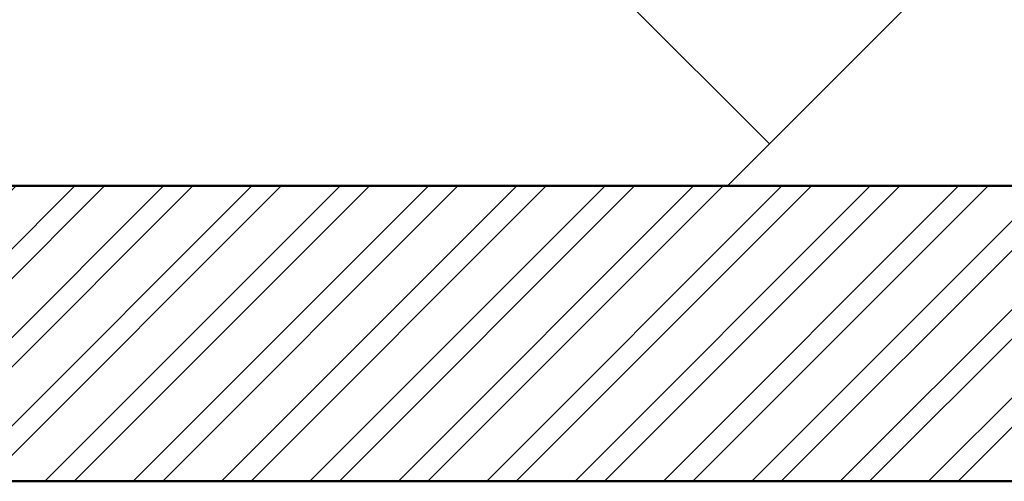
# Model space of a CAD drawing. Units: inches. Extents: x 3590 to 5167, y 65 to 1917.
# Tile 38 of 100: x 5035 to 5065, y 1326 to 1340. Entities that reach past the tile are written whole.
import ezdxf

# ---------------------------------------------------------------- set-up
doc = ezdxf.new("R2010")
doc.units = ezdxf.units.IN
for name, color, linetype, lineweight in [('A-FLOR-PATT', 8, 'Continuous', 13), ('A-WALL', 7, 'Continuous', 50), ('A-WALL-PATT', 251, 'Continuous', 13)]:
    doc.layers.add(name, color=color, linetype=linetype, lineweight=lineweight)

msp = doc.modelspace()

# ---------------------------------------------------------------- hatches: boundary and pattern name
at = {"layer": 'A-FLOR-PATT', "transparency": 33554687}
h = msp.add_hatch(dxfattribs=at)
h.set_pattern_fill('AR-HBONE', color=256, scale=0.2)
h.set_pattern_definition([(45, (-588.972, 0), (0, 28.73682), [60.96, -20.32]), (135, (-574.604, 14.368), (3e-15, 28.73682), [60.96, -20.32])])
h.paths.add_polyline_path([(5071.274, 1796.999), (4933.274, 1796.999), (4933.274, 1753.999), (4962.774, 1753.999, -0.414214), (4928.774, 1719.999), (4933.274, 1718.999), (4933.274, 1334.999), (5071.274, 1334.999)])
h.paths.add_polyline_path([(4951.78, 1521.077), (4951.715, 1521.04), (4951.563, 1520.895)], flags=16)
h.paths.add_polyline_path([(4952.267, 1521.376), (4952.198, 1521.371), (4952.198, 1521.356)], flags=0)
h.paths.add_polyline_path([(4967.051, 1529.728), (4965.231, 1528.694), (4963.411, 1527.714), (4961.756, 1526.851), (4963.589, 1527.449), (4964.036, 1527.478), (4962.975, 1527.249), (4961.76, 1526.852), (4959.792, 1525.834), (4958.005, 1524.895), (4956.24, 1523.93), (4954.504, 1522.919), (4954.129, 1522.682), (4953.361, 1521.997), (4953.366, 1521.998), (4953.605, 1522.064), (4955.106, 1522.761), (4956.921, 1523.434), (4958.678, 1523.915), (4960.358, 1524.2), (4961.945, 1524.286), (4964.171, 1524.108), (4965.958, 1523.309), (4963.863, 1522.976), (4965.187, 1522.499), (4963.366, 1522.497), (4961.545, 1522.487), (4959.764, 1522.461), (4958.304, 1522.419), (4957.974, 1522.388), (4956.307, 1522.232), (4954.718, 1522.071), (4953.251, 1521.899), (4953.525, 1521.623), (4954.331, 1521.379), (4956.243, 1521.23), (4958.039, 1520.93), (4959.684, 1520.483), (4961.16, 1519.896), (4963.107, 1518.8), (4964.393, 1517.325), (4962.973, 1517.726), (4964.558, 1516.661), (4965.407, 1515.708), (4963.507, 1516.322), (4961.68, 1517.005), (4959.935, 1517.745), (4958.282, 1518.528), (4956.732, 1519.343), (4955.295, 1520.175), (4954.672, 1520.572), (4954.513, 1520.627), (4955.658, 1519.318), (4956.703, 1517.982), (4957.644, 1516.647), (4958.485, 1515.334), (4959.55, 1513.524), (4960.438, 1511.769), (4958.841, 1513.62), (4957.452, 1515.325), (4955.819, 1517.459), (4956.665, 1515.448), (4957.111, 1513.923), (4957.447, 1511.714), (4957.076, 1509.793), (4956.538, 1511.11), (4955.992, 1512.569), (4955.444, 1514.125), (4954.898, 1515.735), (4954.357, 1517.356), (4953.824, 1518.943), (4953.305, 1520.452), (4953.065, 1521.116), (4952.971, 1521.146), (4952.949, 1521.086), (4952.73, 1520.199), (4953.37, 1518.024), (4953.757, 1516.373), (4954.051, 1514.765), (4954.264, 1513.221), (4954.471, 1511.131), (4954.497, 1510.402), (4954.409, 1511.76), (4954.264, 1513.221), (4954.051, 1514.765), (4953.757, 1516.373), (4953.37, 1518.024), (4952.877, 1519.698), (4952.716, 1520.141), (4952.533, 1519.059), (4952.374, 1517.789), (4952.219, 1516.312), (4952.046, 1514.6), (4951.833, 1512.626), (4951.557, 1510.363), (4951.203, 1512.168), (4950.852, 1514.339), (4950.985, 1516.376), (4951.66, 1518.286), (4952.593, 1520.481), (4952.357, 1521.13), (4951.855, 1520.328), (4950.839, 1518.908), (4949.777, 1517.587), (4948.916, 1516.617), (4948.111, 1515.256), (4947.089, 1513.554), (4945.889, 1511.615), (4946.326, 1513.402), (4946.562, 1514.249), (4945.528, 1513.327), (4944.581, 1512.531), (4946.018, 1514.508), (4947.204, 1516.048), (4947.893, 1517.313), (4949.307, 1518.764), (4950.414, 1519.767), (4950.451, 1519.806), (4952.267, 1521.376), (4951.645, 1521.493), (4950.404, 1521.18), (4948.044, 1520.359), (4946.119, 1519.452), (4944.572, 1518.475), (4943.35, 1517.443), (4941.997, 1515.92), (4941.661, 1515.275), (4942.813, 1516.99), (4944.572, 1518.475), (4946.119, 1519.452), (4948.044, 1520.359), (4950.404, 1521.18), (4951.645, 1521.493), (4949.647, 1521.868), (4948.6, 1521.756), (4947.126, 1521.57), (4945.42, 1521.348), (4943.45, 1521.105), (4941.183, 1520.856), (4942.86, 1521.613), (4943.873, 1522.03), (4942.952, 1521.909), (4941.41, 1521.485), (4939.543, 1520.67), (4938.968, 1520.226), (4940.733, 1521.299), (4942.952, 1521.909), (4943.702, 1522.008), (4945.894, 1522.7), (4947.565, 1522.714), (4948.921, 1522.566), (4951.131, 1522.183), (4950.971, 1522.297), (4948.129, 1523.006), (4946.035, 1523.707), (4944.232, 1524.521), (4942.707, 1525.461), (4941.444, 1526.537), (4940.43, 1527.761), (4939.649, 1529.143), (4941.421, 1528.122), (4943.147, 1527.132), (4944.841, 1526.175), (4946.514, 1525.25), (4948.179, 1524.359), (4948.365, 1524.263), (4946.475, 1526.045), (4945.181, 1527.54), (4944.19, 1529.033), (4943.496, 1530.54), (4943.278, 1531.36), (4942.498, 1531.919), (4943.114, 1531.762), (4942.959, 1533.659), (4944.14, 1531.989), (4944.612, 1531.323), (4946.202, 1530.463), (4947.486, 1529.509), (4948.79, 1528.226), (4950.368, 1526.237), (4949.485, 1528.155), (4948.851, 1530.123), (4948.491, 1532.041), (4948.381, 1533.918), (4948.501, 1535.76), (4948.827, 1537.573), (4949.418, 1535.565), (4949.957, 1533.569), (4950.464, 1531.586), (4950.961, 1529.617), (4951.391, 1527.954), (4951.724, 1530.687), (4952.201, 1532.58), (4952.889, 1534.33), (4953.77, 1535.951), (4954.827, 1537.46), (4954.521, 1535.39), (4954.273, 1533.937), (4955.58, 1535.663), (4956.748, 1536.739), (4956.159, 1534.78), (4955.589, 1532.873), (4955.043, 1531.006), (4954.525, 1529.166), (4954.038, 1527.341), (4953.638, 1525.733), (4953.611, 1525.586), (4953.398, 1524.166), (4953.382, 1524.009), (4954.07, 1525.476), (4954.912, 1527.022), (4956.136, 1528.894), (4957.847, 1530.577), (4959.376, 1531.54), (4958.256, 1530.104), (4957.143, 1528.663), (4956.066, 1527.243), (4955.056, 1525.871), (4954.141, 1524.571), (4953.352, 1523.372), (4953.311, 1523.303), (4953.273, 1522.925), (4953.261, 1522.382), (4954.103, 1523.373), (4954.63, 1524.284), (4955.961, 1526.358), (4957.23, 1528.13), (4958.421, 1529.609), (4960.037, 1531.368), (4961.374, 1532.375), (4962.101, 1532.77), (4961.07, 1531.061), (4959.987, 1529.438), (4958.869, 1527.908), (4958.15, 1527.007), (4959.803, 1528.003), (4961.589, 1528.793), (4963.391, 1529.328), (4965.211, 1529.632)], flags=16)
h.paths.add_polyline_path([(4962.944, 1523.182), (4961.107, 1523.422), (4960.392, 1523.362), (4962.35, 1523.331)], flags=0)
h.paths.add_polyline_path([(5049.541, 1584.551), (5049.476, 1584.515), (5049.325, 1584.37)], flags=16)
h.paths.add_polyline_path([(5050.028, 1584.851), (5049.959, 1584.845), (5049.959, 1584.83)], flags=0)
h.paths.add_polyline_path([(5042.333, 1581.949), (5043.88, 1582.926), (5045.806, 1583.833), (5048.165, 1584.654), (5049.406, 1584.967), (5047.408, 1585.342), (5046.361, 1585.231), (5044.888, 1585.044), (5043.181, 1584.822), (5041.211, 1584.579), (5038.944, 1584.33), (5040.622, 1585.087), (5041.634, 1585.504), (5040.713, 1585.383), (5039.171, 1584.959), (5037.304, 1584.144), (5036.729, 1583.7), (5038.494, 1584.773), (5040.713, 1585.383), (5041.463, 1585.482), (5043.655, 1586.174), (5045.326, 1586.188), (5046.682, 1586.04), (5048.893, 1585.657), (5048.732, 1585.771), (5045.891, 1586.48), (5043.796, 1587.181), (5041.994, 1587.996), (5040.468, 1588.935), (5039.205, 1590.011), (5038.191, 1591.235), (5037.41, 1592.617), (5039.182, 1591.596), (5040.909, 1590.607), (5042.602, 1589.649), (5044.275, 1588.724), (5045.94, 1587.833), (5046.126, 1587.738), (5044.237, 1589.519), (5042.942, 1591.015), (5041.952, 1592.508), (5041.257, 1594.014), (5041.039, 1594.834), (5040.26, 1595.393), (5040.875, 1595.237), (5040.721, 1597.133), (5041.901, 1595.463), (5042.373, 1594.798), (5043.963, 1593.938), (5045.247, 1592.983), (5046.552, 1591.701), (5048.129, 1589.712), (5047.247, 1591.63), (5046.613, 1593.597), (5046.252, 1595.515), (5046.142, 1597.392), (5046.262, 1599.234), (5046.588, 1601.047), (5047.179, 1599.039), (5047.718, 1597.043), (5048.225, 1595.06), (5048.722, 1593.091), (5049.152, 1591.429), (5049.485, 1594.161), (5049.962, 1596.054), (5050.65, 1597.804), (5051.532, 1599.425), (5052.589, 1600.934), (5052.283, 1598.864), (5052.034, 1597.411), (5053.341, 1599.137), (5054.509, 1600.213), (5053.92, 1598.254), (5053.35, 1596.348), (5052.805, 1594.48), (5052.286, 1592.64), (5051.799, 1590.815), (5051.4, 1589.207), (5051.373, 1589.06), (5051.159, 1587.64), (5051.143, 1587.483), (5051.831, 1588.95), (5052.673, 1590.496), (5053.898, 1592.368), (5055.608, 1594.051), (5057.137, 1595.014), (5056.017, 1593.578), (5054.904, 1592.137), (5053.828, 1590.717), (5052.817, 1589.345), (5051.902, 1588.046), (5051.113, 1586.846), (5051.072, 1586.777), (5051.034, 1586.399), (5051.022, 1585.856), (5051.864, 1586.847), (5052.391, 1587.758), (5053.723, 1589.832), (5054.991, 1591.604), (5056.182, 1593.083), (5057.798, 1594.842), (5059.135, 1595.849), (5059.863, 1596.244), (5058.831, 1594.535), (5057.749, 1592.912), (5056.63, 1591.382), (5055.912, 1590.482), (5057.564, 1591.477), (5059.35, 1592.267), (5061.152, 1592.802), (5062.972, 1593.106), (5064.812, 1593.203), (5062.992, 1592.169), (5061.172, 1591.188), (5059.518, 1590.325), (5061.35, 1590.924), (5061.797, 1590.952), (5060.737, 1590.723), (5059.521, 1590.326), (5057.553, 1589.308), (5055.766, 1588.369), (5054.002, 1587.404), (5052.265, 1586.393), (5051.891, 1586.156), (5051.122, 1585.471), (5051.127, 1585.472), (5051.366, 1585.538), (5052.867, 1586.235), (5054.682, 1586.908), (5056.439, 1587.389), (5058.12, 1587.675), (5059.706, 1587.76), (5061.933, 1587.583), (5063.719, 1586.783), (5061.624, 1586.45), (5062.949, 1585.973), (5061.127, 1585.971), (5059.307, 1585.961), (5057.525, 1585.935), (5056.065, 1585.893), (5055.735, 1585.862), (5054.068, 1585.707), (5052.479, 1585.546), (5051.012, 1585.373), (5051.286, 1585.097), (5052.092, 1584.853), (5054.004, 1584.704), (5055.8, 1584.404), (5057.446, 1583.958), (5058.921, 1583.37), (5060.868, 1582.274), (5062.154, 1580.799), (5060.734, 1581.2), (5062.32, 1580.135), (5063.168, 1579.182), (5061.269, 1579.796), (5059.441, 1580.479), (5057.696, 1581.219), (5056.043, 1582.003), (5054.493, 1582.817), (5053.057, 1583.649), (5052.433, 1584.047), (5052.274, 1584.101), (5053.42, 1582.793), (5054.464, 1581.457), (5055.405, 1580.121), (5056.247, 1578.809), (5057.311, 1576.998), (5058.199, 1575.244), (5056.602, 1577.094), (5055.213, 1578.799), (5053.58, 1580.933), (5054.427, 1578.922), (5054.872, 1577.397), (5055.208, 1575.189), (5054.838, 1573.267), (5054.299, 1574.584), (5053.754, 1576.043), (5053.206, 1577.599), (5052.659, 1579.209), (5052.118, 1580.83), (5051.585, 1582.417), (5051.066, 1583.927), (5050.826, 1584.59), (5050.733, 1584.62), (5050.711, 1584.561), (5050.491, 1583.673), (5051.131, 1581.498), (5051.518, 1579.847), (5051.813, 1578.24), (5052.026, 1576.695), (5052.233, 1574.605), (5052.258, 1573.876), (5052.17, 1575.234), (5052.026, 1576.695), (5051.813, 1578.24), (5051.518, 1579.847), (5051.131, 1581.498), (5050.638, 1583.172), (5050.477, 1583.615), (5050.294, 1582.533), (5050.136, 1581.263), (5049.981, 1579.786), (5049.807, 1578.074), (5049.594, 1576.1), (5049.318, 1573.837), (5048.965, 1575.642), (5048.613, 1577.813), (5048.747, 1579.85), (5049.421, 1581.76), (5050.354, 1583.955), (5050.118, 1584.604), (5049.616, 1583.802), (5048.6, 1582.382), (5047.538, 1581.061), (5046.677, 1580.091), (5045.872, 1578.73), (5044.85, 1577.028), (5043.651, 1575.089), (5044.087, 1576.877), (5044.324, 1577.723), (5043.289, 1576.801), (5042.342, 1576.005), (5043.779, 1577.982), (5044.966, 1579.522), (5045.655, 1580.787), (5047.068, 1582.239), (5048.175, 1583.241), (5048.213, 1583.28), (5050.028, 1584.851), (5049.406, 1584.967), (5048.165, 1584.654), (5045.806, 1583.833), (5043.88, 1582.926), (5042.333, 1581.949), (5041.111, 1580.917), (5039.758, 1579.394), (5039.423, 1578.749), (5040.575, 1580.464)], flags=16)
h.paths.add_polyline_path([(4954.799, 1533.12), (4954.262, 1532.079), (4953.831, 1530.935), (4953.505, 1529.636), (4953.283, 1528.133), (4953.167, 1526.376), (4953.156, 1524.315), (4953.277, 1521.236), (4952.802, 1521.842), (4951.557, 1521.998), (4950.976, 1521.961), (4952.661, 1521.941), (4952.802, 1521.842), (4953.152, 1523.593), (4953.167, 1526.376), (4953.283, 1528.133), (4953.609, 1530.346), (4954.456, 1532.592)], flags=0)
h.paths.add_polyline_path([(5050.563, 1585.316), (5049.318, 1585.472), (5048.737, 1585.435), (5050.422, 1585.415), (5050.563, 1585.316), (5050.914, 1587.067), (5050.928, 1589.851), (5051.045, 1591.607), (5051.371, 1593.82), (5052.217, 1596.066), (5052.56, 1596.594), (5052.024, 1595.554), (5051.592, 1594.409), (5051.266, 1593.11), (5051.045, 1591.607), (5050.928, 1589.851), (5050.918, 1587.789), (5051.038, 1584.71)], flags=0)
h.paths.add_polyline_path([(5058.153, 1586.836), (5060.111, 1586.805), (5060.705, 1586.656), (5058.868, 1586.896)], flags=0)
h.paths.add_polyline_path([(5049.541, 1430.936), (5049.476, 1430.9), (5049.325, 1430.755)], flags=16)
h.paths.add_polyline_path([(5050.028, 1431.236), (5049.959, 1431.231), (5049.959, 1431.215)], flags=0)
h.paths.add_polyline_path([(5046.588, 1447.432), (5047.179, 1445.425), (5047.718, 1443.429), (5048.225, 1441.446), (5048.722, 1439.476), (5049.152, 1437.814), (5049.485, 1440.546), (5049.962, 1442.439), (5050.65, 1444.189), (5051.532, 1445.811), (5052.589, 1447.319), (5052.283, 1445.249), (5052.034, 1443.796), (5053.341, 1445.522), (5054.509, 1446.598), (5053.92, 1444.64), (5053.35, 1442.733), (5052.805, 1440.865), (5052.286, 1439.025), (5051.799, 1437.201), (5051.4, 1435.592), (5051.373, 1435.445), (5051.159, 1434.025), (5051.143, 1433.868), (5051.831, 1435.335), (5052.673, 1436.881), (5053.898, 1438.753), (5055.608, 1440.436), (5057.137, 1441.4), (5056.017, 1439.963), (5054.904, 1438.522), (5053.828, 1437.102), (5052.817, 1435.73), (5051.902, 1434.431), (5051.113, 1433.231), (5051.072, 1433.162), (5051.034, 1432.784), (5051.022, 1432.242), (5051.864, 1433.232), (5052.391, 1434.143), (5053.723, 1436.217), (5054.991, 1437.989), (5056.182, 1439.468), (5057.798, 1441.227), (5059.135, 1442.235), (5059.863, 1442.629), (5058.831, 1440.921), (5057.749, 1439.298), (5056.63, 1437.767), (5055.912, 1436.867), (5057.564, 1437.863), (5059.35, 1438.652), (5061.152, 1439.187), (5062.972, 1439.491), (5064.812, 1439.588), (5062.992, 1438.554), (5061.172, 1437.573), (5059.518, 1436.71), (5061.35, 1437.309), (5061.797, 1437.337), (5060.737, 1437.108), (5059.521, 1436.711), (5057.553, 1435.693), (5055.766, 1434.754), (5054.002, 1433.789), (5052.265, 1432.778), (5051.891, 1432.541), (5051.122, 1431.856), (5051.127, 1431.857), (5051.366, 1431.923), (5052.867, 1432.62), (5054.682, 1433.293), (5056.439, 1433.775), (5058.12, 1434.06), (5059.706, 1434.145), (5061.933, 1433.968), (5063.719, 1433.168), (5061.624, 1432.835), (5062.949, 1432.358), (5061.127, 1432.357), (5059.307, 1432.346), (5057.525, 1432.32), (5056.065, 1432.278), (5055.735, 1432.248), (5054.068, 1432.092), (5052.479, 1431.931), (5051.012, 1431.759), (5051.286, 1431.482), (5052.092, 1431.238), (5054.004, 1431.089), (5055.8, 1430.789), (5057.446, 1430.343), (5058.921, 1429.755), (5060.868, 1428.66), (5062.154, 1427.185), (5060.734, 1427.585), (5062.32, 1426.52), (5063.168, 1425.567), (5061.269, 1426.181), (5059.441, 1426.865), (5057.696, 1427.604), (5056.043, 1428.388), (5054.493, 1429.202), (5053.057, 1430.034), (5052.433, 1430.432), (5052.274, 1430.487), (5053.42, 1429.178), (5054.464, 1427.842), (5055.405, 1426.506), (5056.247, 1425.194), (5057.311, 1423.383), (5058.199, 1421.629), (5056.602, 1423.479), (5055.213, 1425.184), (5053.58, 1427.318), (5054.427, 1425.307), (5054.872, 1423.782), (5055.208, 1421.574), (5054.838, 1419.652), (5054.299, 1420.97), (5053.754, 1422.428), (5053.206, 1423.984), (5052.659, 1425.595), (5052.118, 1427.215), (5051.585, 1428.802), (5051.066, 1430.312), (5050.826, 1430.975), (5050.733, 1431.005), (5050.711, 1430.946), (5050.491, 1430.058), (5051.131, 1427.883), (5051.518, 1426.232), (5051.813, 1424.625), (5052.026, 1423.081), (5052.233, 1420.991), (5052.258, 1420.261), (5052.17, 1421.619), (5052.026, 1423.081), (5051.813, 1424.625), (5051.518, 1426.232), (5051.131, 1427.883), (5050.638, 1429.558), (5050.477, 1430.001), (5050.294, 1428.918), (5050.136, 1427.648), (5049.981, 1426.171), (5049.807, 1424.459), (5049.594, 1422.485), (5049.318, 1420.222), (5048.965, 1422.028), (5048.613, 1424.199), (5048.747, 1426.235), (5049.421, 1428.146), (5050.354, 1430.34), (5050.118, 1430.989), (5049.616, 1430.187), (5048.6, 1428.768), (5047.538, 1427.446), (5046.677, 1426.477), (5045.872, 1425.116), (5044.85, 1423.413), (5043.651, 1421.474), (5044.087, 1423.262), (5044.324, 1424.109), (5043.289, 1423.186), (5042.342, 1422.391), (5043.779, 1424.368), (5044.966, 1425.907), (5045.655, 1427.173), (5047.068, 1428.624), (5048.175, 1429.627), (5048.213, 1429.666), (5050.028, 1431.236), (5049.406, 1431.353), (5048.165, 1431.039), (5045.806, 1430.218), (5043.88, 1429.311), (5042.333, 1428.334), (5041.111, 1427.302), (5039.758, 1425.779), (5039.423, 1425.134), (5040.575, 1426.849), (5042.333, 1428.334), (5043.88, 1429.311), (5045.806, 1430.218), (5048.165, 1431.039), (5049.406, 1431.353), (5047.408, 1431.727), (5046.361, 1431.616), (5044.888, 1431.429), (5043.181, 1431.207), (5041.211, 1430.964), (5038.944, 1430.715), (5040.622, 1431.472), (5041.634, 1431.89), (5040.713, 1431.769), (5039.171, 1431.345), (5037.304, 1430.53), (5036.729, 1430.085), (5038.494, 1431.158), (5040.713, 1431.769), (5041.463, 1431.867), (5043.655, 1432.559), (5045.326, 1432.573), (5046.682, 1432.425), (5048.893, 1432.042), (5048.732, 1432.156), (5045.891, 1432.865), (5043.796, 1433.566), (5041.994, 1434.381), (5040.468, 1435.321), (5039.205, 1436.396), (5038.191, 1437.62), (5037.41, 1439.002), (5039.182, 1437.982), (5040.909, 1436.992), (5042.602, 1436.034), (5044.275, 1435.109), (5045.94, 1434.218), (5046.126, 1434.123), (5044.237, 1435.904), (5042.942, 1437.4), (5041.952, 1438.893), (5041.257, 1440.399), (5041.039, 1441.219), (5040.26, 1441.778), (5040.875, 1441.622), (5040.721, 1443.518), (5041.901, 1441.848), (5042.373, 1441.183), (5043.963, 1440.323), (5045.247, 1439.369), (5046.552, 1438.086), (5048.129, 1436.097), (5047.247, 1438.015), (5046.613, 1439.982), (5046.252, 1441.901), (5046.142, 1443.778), (5046.262, 1445.619)], flags=16)
h.paths.add_polyline_path([(5052.382, 1444.255), (5051.623, 1442.78), (5052.024, 1441.939), (5052.56, 1442.98)], flags=0)
h.paths.add_polyline_path([(5050.563, 1431.701), (5049.318, 1431.857), (5048.737, 1431.821), (5050.422, 1431.8)], flags=0)
h.paths.add_polyline_path([(5058.153, 1433.221), (5060.111, 1433.19), (5060.705, 1433.041), (5058.868, 1433.281)], flags=0)
h.paths.add_polyline_path([(5049.541, 1352.285), (5049.476, 1352.249), (5049.325, 1352.104)], flags=16)
h.paths.add_polyline_path([(5050.028, 1352.585), (5049.959, 1352.58), (5049.959, 1352.564)], flags=0)
h.paths.add_polyline_path([(5046.588, 1368.781), (5047.179, 1366.774), (5047.718, 1364.778), (5048.225, 1362.795), (5048.722, 1360.825), (5049.152, 1359.163), (5049.485, 1361.896), (5049.962, 1363.789), (5050.65, 1365.538), (5051.532, 1367.16), (5052.589, 1368.669), (5052.283, 1366.598), (5052.034, 1365.145), (5053.341, 1366.871), (5054.509, 1367.947), (5053.92, 1365.989), (5053.35, 1364.082), (5052.805, 1362.214), (5052.286, 1360.374), (5051.799, 1358.55), (5051.4, 1356.942), (5051.373, 1356.794), (5051.159, 1355.374), (5051.143, 1355.218), (5051.831, 1356.684), (5052.673, 1358.23), (5053.898, 1360.102), (5055.608, 1361.786), (5057.137, 1362.749), (5056.017, 1361.313), (5054.904, 1359.872), (5053.828, 1358.452), (5052.817, 1357.079), (5051.902, 1355.78), (5051.113, 1354.581), (5051.072, 1354.512), (5051.034, 1354.133), (5051.022, 1353.591), (5051.864, 1354.581), (5052.391, 1355.492), (5053.723, 1357.566), (5054.991, 1359.338), (5056.182, 1360.817), (5057.798, 1362.577), (5059.135, 1363.584), (5059.863, 1363.979), (5058.831, 1362.27), (5057.749, 1360.647), (5056.63, 1359.117), (5055.912, 1358.216), (5057.564, 1359.212), (5059.35, 1360.001), (5061.152, 1360.536), (5062.972, 1360.841), (5064.812, 1360.937), (5062.992, 1359.903), (5061.172, 1358.923), (5059.518, 1358.059), (5061.35, 1358.658), (5061.797, 1358.687), (5060.737, 1358.458), (5059.521, 1358.061), (5057.553, 1357.043), (5055.766, 1356.103), (5054.002, 1355.138), (5052.265, 1354.127), (5051.891, 1353.89), (5051.122, 1353.206), (5051.127, 1353.206), (5051.366, 1353.272), (5052.867, 1353.969), (5054.682, 1354.643), (5056.439, 1355.124), (5058.12, 1355.409), (5059.706, 1355.495), (5061.933, 1355.317), (5063.719, 1354.518), (5061.624, 1354.184), (5062.949, 1353.708), (5061.127, 1353.706), (5059.307, 1353.695), (5057.525, 1353.669), (5056.065, 1353.627), (5055.735, 1353.597), (5054.068, 1353.441), (5052.479, 1353.28), (5051.012, 1353.108), (5051.286, 1352.831), (5052.092, 1352.587), (5054.004, 1352.439), (5055.8, 1352.138), (5057.446, 1351.692), (5058.921, 1351.104), (5060.868, 1350.009), (5062.154, 1348.534), (5060.734, 1348.935), (5062.32, 1347.869), (5063.168, 1346.916), (5061.269, 1347.53), (5059.441, 1348.214), (5057.696, 1348.954), (5056.043, 1349.737), (5054.493, 1350.551), (5053.057, 1351.383), (5052.433, 1351.781), (5052.274, 1351.836), (5053.42, 1350.527), (5054.464, 1349.191), (5055.405, 1347.855), (5056.247, 1346.543), (5057.311, 1344.733), (5058.199, 1342.978), (5056.602, 1344.828), (5055.213, 1346.534), (5053.58, 1348.667), (5054.427, 1346.656), (5054.872, 1345.132), (5055.208, 1342.923), (5054.838, 1341.002), (5054.299, 1342.319), (5053.754, 1343.778), (5053.206, 1345.334), (5052.659, 1346.944), (5052.118, 1348.564), (5051.585, 1350.151), (5051.066, 1351.661), (5050.826, 1352.324), (5050.733, 1352.355), (5050.711, 1352.295), (5050.491, 1351.408), (5051.131, 1349.232), (5051.518, 1347.581), (5051.813, 1345.974), (5052.026, 1344.43), (5052.233, 1342.34), (5052.258, 1341.61), (5052.17, 1342.969), (5052.026, 1344.43), (5051.813, 1345.974), (5051.518, 1347.581), (5051.131, 1349.232), (5050.638, 1350.907), (5050.477, 1351.35), (5050.294, 1350.267), (5050.136, 1348.997), (5049.981, 1347.52), (5049.807, 1345.809), (5049.594, 1343.835), (5049.318, 1341.571), (5048.965, 1343.377), (5048.613, 1345.548), (5048.747, 1347.585), (5049.421, 1349.495), (5050.354, 1351.689), (5050.118, 1352.339), (5049.616, 1351.536), (5048.6, 1350.117), (5047.538, 1348.795), (5046.677, 1347.826), (5045.872, 1346.465), (5044.85, 1344.763), (5043.651, 1342.824), (5044.087, 1344.611), (5044.324, 1345.458), (5043.289, 1344.535), (5042.342, 1343.74), (5043.779, 1345.717), (5044.966, 1347.256), (5045.655, 1348.522), (5047.068, 1349.973), (5048.175, 1350.976), (5048.213, 1351.015), (5050.028, 1352.585), (5049.406, 1352.702), (5048.165, 1352.388), (5045.806, 1351.567), (5043.88, 1350.661), (5042.333, 1349.683), (5041.111, 1348.651), (5039.758, 1347.128), (5039.423, 1346.483), (5040.575, 1348.198), (5042.333, 1349.683), (5043.88, 1350.661), (5045.806, 1351.567), (5048.165, 1352.388), (5049.406, 1352.702), (5047.408, 1353.076), (5046.361, 1352.965), (5044.888, 1352.779), (5043.181, 1352.556), (5041.211, 1352.313), (5038.944, 1352.065), (5040.622, 1352.821), (5041.634, 1353.239), (5040.713, 1353.118), (5039.171, 1352.694), (5037.304, 1351.879), (5036.729, 1351.434), (5038.494, 1352.508), (5040.713, 1353.118), (5041.463, 1353.216), (5043.655, 1353.909), (5045.326, 1353.923), (5046.682, 1353.774), (5048.893, 1353.391), (5048.732, 1353.506), (5045.891, 1354.214), (5043.796, 1354.915), (5041.994, 1355.73), (5040.468, 1356.67), (5039.205, 1357.746), (5038.191, 1358.969), (5037.41, 1360.352), (5039.182, 1359.331), (5040.909, 1358.341), (5042.602, 1357.383), (5044.275, 1356.458), (5045.94, 1355.567), (5046.126, 1355.472), (5044.237, 1357.253), (5042.942, 1358.749), (5041.952, 1360.242), (5041.257, 1361.748), (5041.039, 1362.568), (5040.26, 1363.128), (5040.875, 1362.971), (5040.721, 1364.867), (5041.901, 1363.197), (5042.373, 1362.532), (5043.963, 1361.672), (5045.247, 1360.718), (5046.552, 1359.435), (5048.129, 1357.446), (5047.247, 1359.364), (5046.613, 1361.331), (5046.252, 1363.25), (5046.142, 1365.127), (5046.262, 1366.969)], flags=16)
h.paths.add_polyline_path([(5052.382, 1365.604), (5051.623, 1364.129), (5052.024, 1363.288), (5052.56, 1364.329)], flags=0)
h.paths.add_polyline_path([(4951.78, 1698.041), (4951.715, 1698.005), (4951.563, 1697.859)], flags=16)
h.paths.add_polyline_path([(4952.267, 1698.341), (4952.198, 1698.335), (4952.198, 1698.32)], flags=0)
h.paths.add_polyline_path([(4957.076, 1686.757), (4956.538, 1688.074), (4955.992, 1689.533), (4955.444, 1691.089), (4954.898, 1692.699), (4954.357, 1694.32), (4953.824, 1695.907), (4953.305, 1697.417), (4953.065, 1698.08), (4952.971, 1698.11), (4952.949, 1698.051), (4952.73, 1697.163), (4953.37, 1694.988), (4953.757, 1693.337), (4954.051, 1691.729), (4954.264, 1690.185), (4954.471, 1688.095), (4954.497, 1687.366), (4954.409, 1688.724), (4954.264, 1690.185), (4954.051, 1691.729), (4953.757, 1693.337), (4953.37, 1694.988), (4952.877, 1696.662), (4952.716, 1697.105), (4952.533, 1696.023), (4952.374, 1694.753), (4952.219, 1693.276), (4952.046, 1691.564), (4951.833, 1689.59), (4951.557, 1687.327), (4951.203, 1689.132), (4950.852, 1691.303), (4950.985, 1693.34), (4951.66, 1695.25), (4952.593, 1697.445), (4952.357, 1698.094), (4951.855, 1697.292), (4950.839, 1695.872), (4949.777, 1694.551), (4948.916, 1693.581), (4948.111, 1692.22), (4947.089, 1690.518), (4945.889, 1688.579), (4946.326, 1690.366), (4946.562, 1691.213), (4945.528, 1690.291), (4944.581, 1689.495), (4946.018, 1691.472), (4947.204, 1693.012), (4947.893, 1694.277), (4949.307, 1695.729), (4950.414, 1696.731), (4950.451, 1696.77), (4952.267, 1698.341), (4951.645, 1698.457), (4950.404, 1698.144), (4948.044, 1697.323), (4946.119, 1696.416), (4944.572, 1695.439), (4943.35, 1694.407), (4941.997, 1692.884), (4941.661, 1692.239), (4942.813, 1693.954), (4944.572, 1695.439), (4946.119, 1696.416), (4948.044, 1697.323), (4950.404, 1698.144), (4951.645, 1698.457), (4949.647, 1698.832), (4948.6, 1698.72), (4947.126, 1698.534), (4945.42, 1698.312), (4943.45, 1698.069), (4941.183, 1697.82), (4942.86, 1698.577), (4943.873, 1698.994), (4942.952, 1698.873), (4941.41, 1698.449), (4939.543, 1697.634), (4938.968, 1697.19), (4940.733, 1698.263), (4942.952, 1698.873), (4943.702, 1698.972), (4945.894, 1699.664), (4947.565, 1699.678), (4948.921, 1699.53), (4951.131, 1699.147), (4950.971, 1699.261), (4948.129, 1699.97), (4946.035, 1700.671), (4944.232, 1701.486), (4942.707, 1702.425), (4941.444, 1703.501), (4940.43, 1704.725), (4939.649, 1706.107), (4941.421, 1705.086), (4943.147, 1704.097), (4944.841, 1703.139), (4946.514, 1702.214), (4948.179, 1701.323), (4948.365, 1701.227), (4946.475, 1703.009), (4945.181, 1704.505), (4944.19, 1705.997), (4943.496, 1707.504), (4943.278, 1708.324), (4942.498, 1708.883), (4943.114, 1708.727), (4942.959, 1710.623), (4944.14, 1708.953), (4944.612, 1708.287), (4946.202, 1707.428), (4947.486, 1706.473), (4948.79, 1705.191), (4950.368, 1703.202), (4949.485, 1705.12), (4948.851, 1707.087), (4948.491, 1709.005), (4948.381, 1710.882), (4948.501, 1712.724), (4948.827, 1714.537), (4949.418, 1712.529), (4949.957, 1710.533), (4950.464, 1708.55), (4950.961, 1706.581), (4951.391, 1704.919), (4951.724, 1707.651), (4952.201, 1709.544), (4952.889, 1711.294), (4953.77, 1712.915), (4954.827, 1714.424), (4954.521, 1712.354), (4954.273, 1710.901), (4955.58, 1712.627), (4956.748, 1713.703), (4956.159, 1711.744), (4955.589, 1709.837), (4955.043, 1707.97), (4954.525, 1706.13), (4954.038, 1704.305), (4953.638, 1702.697), (4953.611, 1702.55), (4953.398, 1701.13), (4953.382, 1700.973), (4954.07, 1702.44), (4954.912, 1703.986), (4956.136, 1705.858), (4957.847, 1707.541), (4959.376, 1708.504), (4958.256, 1707.068), (4957.143, 1705.627), (4956.066, 1704.207), (4955.056, 1702.835), (4954.141, 1701.536), (4953.352, 1700.336), (4953.311, 1700.267), (4953.273, 1699.889), (4953.261, 1699.346), (4954.103, 1700.337), (4954.63, 1701.248), (4955.961, 1703.322), (4957.23, 1705.094), (4958.421, 1706.573), (4960.037, 1708.332), (4961.374, 1709.339), (4962.101, 1709.734), (4961.07, 1708.025), (4959.987, 1706.402), (4958.869, 1704.872), (4958.15, 1703.972), (4959.803, 1704.967), (4961.589, 1705.757), (4963.391, 1706.292), (4965.211, 1706.596), (4967.051, 1706.692), (4965.231, 1705.659), (4963.411, 1704.678), (4961.756, 1703.815), (4963.589, 1704.413), (4964.036, 1704.442), (4962.975, 1704.213), (4961.76, 1703.816), (4959.792, 1702.798), (4958.005, 1701.859), (4956.24, 1700.894), (4954.504, 1699.883), (4954.129, 1699.646), (4953.361, 1698.961), (4953.366, 1698.962), (4953.605, 1699.028), (4955.106, 1699.725), (4956.921, 1700.398), (4958.678, 1700.879), (4960.358, 1701.164), (4961.945, 1701.25), (4964.171, 1701.073), (4965.958, 1700.273), (4963.863, 1699.94), (4965.187, 1699.463), (4963.366, 1699.461), (4961.545, 1699.451), (4959.764, 1699.425), (4958.304, 1699.383), (4957.974, 1699.352), (4956.307, 1699.197), (4954.718, 1699.036), (4953.251, 1698.863), (4953.525, 1698.587), (4954.331, 1698.343), (4956.243, 1698.194), (4958.039, 1697.894), (4959.684, 1697.447), (4961.16, 1696.86), (4963.107, 1695.764), (4964.393, 1694.289), (4962.973, 1694.69), (4964.558, 1693.625), (4965.407, 1692.672), (4963.507, 1693.286), (4961.68, 1693.969), (4959.935, 1694.709), (4958.282, 1695.492), (4956.732, 1696.307), (4955.295, 1697.139), (4954.672, 1697.536), (4954.513, 1697.591), (4955.658, 1696.282), (4956.703, 1694.946), (4957.644, 1693.611), (4958.485, 1692.298), (4959.55, 1690.488), (4960.438, 1688.733), (4958.841, 1690.584), (4957.452, 1692.289), (4955.819, 1694.423), (4956.665, 1692.412), (4957.111, 1690.887), (4957.447, 1688.678)], flags=16)
h.paths.add_polyline_path([(5050.563, 1353.05), (5049.318, 1353.207), (5048.737, 1353.17), (5050.422, 1353.15)], flags=0)
h.paths.add_polyline_path([(4951.78, 1351.486), (4951.715, 1351.45), (4951.563, 1351.305)], flags=16)
h.paths.add_polyline_path([(4952.267, 1351.786), (4952.198, 1351.78), (4952.198, 1351.765)], flags=0)
h.paths.add_polyline_path([(4954.827, 1367.869), (4954.521, 1365.799), (4954.273, 1364.346), (4955.58, 1366.072), (4956.748, 1367.148), (4956.159, 1365.19), (4955.589, 1363.283), (4955.043, 1361.415), (4954.525, 1359.575), (4954.038, 1357.751), (4953.638, 1356.142), (4953.611, 1355.995), (4953.398, 1354.575), (4953.382, 1354.418), (4954.07, 1355.885), (4954.912, 1357.431), (4956.136, 1359.303), (4957.847, 1360.986), (4959.376, 1361.95), (4958.256, 1360.513), (4957.143, 1359.072), (4956.066, 1357.652), (4955.056, 1356.28), (4954.141, 1354.981), (4953.352, 1353.781), (4953.311, 1353.712), (4953.273, 1353.334), (4953.261, 1352.792), (4954.103, 1353.782), (4954.63, 1354.693), (4955.961, 1356.767), (4957.23, 1358.539), (4958.421, 1360.018), (4960.037, 1361.777), (4961.374, 1362.785), (4962.101, 1363.179), (4961.07, 1361.471), (4959.987, 1359.848), (4958.869, 1358.317), (4958.15, 1357.417), (4959.803, 1358.413), (4961.589, 1359.202), (4963.391, 1359.737), (4965.211, 1360.041), (4967.051, 1360.138), (4965.231, 1359.104), (4963.411, 1358.123), (4961.756, 1357.26), (4963.589, 1357.859), (4964.036, 1357.887), (4962.975, 1357.658), (4961.76, 1357.261), (4959.792, 1356.243), (4958.005, 1355.304), (4956.24, 1354.339), (4954.504, 1353.328), (4954.129, 1353.091), (4953.361, 1352.406), (4953.366, 1352.407), (4953.605, 1352.473), (4955.106, 1353.17), (4956.921, 1353.843), (4958.678, 1354.325), (4960.358, 1354.61), (4961.945, 1354.695), (4964.171, 1354.518), (4965.958, 1353.718), (4963.863, 1353.385), (4965.187, 1352.908), (4963.366, 1352.907), (4961.545, 1352.896), (4959.764, 1352.87), (4958.304, 1352.828), (4957.974, 1352.798), (4956.307, 1352.642), (4954.718, 1352.481), (4953.251, 1352.309), (4953.525, 1352.032), (4954.331, 1351.788), (4956.243, 1351.639), (4958.039, 1351.339), (4959.684, 1350.893), (4961.16, 1350.305), (4963.107, 1349.21), (4964.393, 1347.735), (4962.973, 1348.135), (4964.558, 1347.07), (4965.407, 1346.117), (4963.507, 1346.731), (4961.68, 1347.414), (4959.935, 1348.154), (4958.282, 1348.938), (4956.732, 1349.752), (4955.295, 1350.584), (4954.672, 1350.982), (4954.513, 1351.036), (4955.658, 1349.728), (4956.703, 1348.392), (4957.644, 1347.056), (4958.485, 1345.744), (4959.55, 1343.933), (4960.438, 1342.179), (4958.841, 1344.029), (4957.452, 1345.734), (4955.819, 1347.868), (4956.665, 1345.857), (4957.111, 1344.332), (4957.447, 1342.124), (4957.076, 1340.202), (4956.538, 1341.52), (4955.992, 1342.978), (4955.444, 1344.534), (4954.898, 1346.145), (4954.357, 1347.765), (4953.824, 1349.352), (4953.305, 1350.862), (4953.065, 1351.525), (4952.971, 1351.555), (4952.949, 1351.496), (4952.73, 1350.608), (4953.37, 1348.433), (4953.757, 1346.782), (4954.051, 1345.175), (4954.264, 1343.631), (4954.471, 1341.541), (4954.497, 1340.811), (4954.409, 1342.169), (4954.264, 1343.631), (4954.051, 1345.175), (4953.757, 1346.782), (4953.37, 1348.433), (4952.877, 1350.108), (4952.716, 1350.551), (4952.533, 1349.468), (4952.374, 1348.198), (4952.219, 1346.721), (4952.046, 1345.009), (4951.833, 1343.035), (4951.557, 1340.772), (4951.203, 1342.578), (4950.852, 1344.749), (4950.985, 1346.785), (4951.66, 1348.696), (4952.593, 1350.89), (4952.357, 1351.539), (4951.855, 1350.737), (4950.839, 1349.318), (4949.777, 1347.996), (4948.916, 1347.027), (4948.111, 1345.665), (4947.089, 1343.963), (4945.889, 1342.024), (4946.326, 1343.812), (4946.562, 1344.659), (4945.528, 1343.736), (4944.581, 1342.941), (4946.018, 1344.918), (4947.204, 1346.457), (4947.893, 1347.723), (4949.307, 1349.174), (4950.414, 1350.177), (4950.451, 1350.216), (4952.267, 1351.786), (4951.645, 1351.903), (4950.404, 1351.589), (4948.044, 1350.768), (4946.119, 1349.861), (4944.572, 1348.884), (4943.35, 1347.852), (4941.997, 1346.329), (4941.661, 1345.684), (4942.813, 1347.399), (4944.572, 1348.884), (4946.119, 1349.861), (4948.044, 1350.768), (4950.404, 1351.589), (4951.645, 1351.903), (4949.647, 1352.277), (4948.6, 1352.166), (4947.126, 1351.979), (4945.42, 1351.757), (4943.45, 1351.514), (4941.183, 1351.265), (4942.86, 1352.022), (4943.873, 1352.44), (4942.952, 1352.319), (4941.41, 1351.895), (4939.543, 1351.08), (4938.968, 1350.635), (4940.733, 1351.708), (4942.952, 1352.319), (4943.702, 1352.417), (4945.894, 1353.109), (4947.565, 1353.123), (4948.921, 1352.975), (4951.131, 1352.592), (4950.971, 1352.706), (4948.129, 1353.415), (4946.035, 1354.116), (4944.232, 1354.931), (4942.707, 1355.871), (4941.444, 1356.946), (4940.43, 1358.17), (4939.649, 1359.552), (4941.421, 1358.532), (4943.147, 1357.542), (4944.841, 1356.584), (4946.514, 1355.659), (4948.179, 1354.768), (4948.365, 1354.673), (4946.475, 1356.454), (4945.181, 1357.95), (4944.19, 1359.443), (4943.496, 1360.949), (4943.278, 1361.769), (4942.498, 1362.328), (4943.114, 1362.172), (4942.959, 1364.068), (4944.14, 1362.398), (4944.612, 1361.733), (4946.202, 1360.873), (4947.486, 1359.919), (4948.79, 1358.636), (4950.368, 1356.647), (4949.485, 1358.565), (4948.851, 1360.532), (4948.491, 1362.451), (4948.381, 1364.328), (4948.501, 1366.169), (4948.827, 1367.982), (4949.418, 1365.975), (4949.957, 1363.979), (4950.464, 1361.995), (4950.961, 1360.026), (4951.391, 1358.364), (4951.724, 1361.096), (4952.201, 1362.989), (4952.889, 1364.739), (4953.77, 1366.361)], flags=16)
h.paths.add_polyline_path([(4954.799, 1363.53), (4954.262, 1362.489), (4953.831, 1361.344), (4953.505, 1360.045), (4953.283, 1358.543), (4953.167, 1356.786), (4953.156, 1354.724), (4953.277, 1351.646), (4952.802, 1352.251), (4951.557, 1352.407), (4950.976, 1352.371), (4952.661, 1352.35), (4952.802, 1352.251), (4953.152, 1354.002), (4953.167, 1356.786), (4953.283, 1358.543), (4953.609, 1360.755), (4954.456, 1363.001)], flags=0)
h.paths.add_polyline_path([(4952.802, 1698.806), (4951.557, 1698.962), (4950.976, 1698.925), (4952.661, 1698.905), (4952.802, 1698.806), (4953.152, 1700.557), (4953.167, 1703.34), (4953.283, 1705.097), (4953.609, 1707.31), (4954.456, 1709.556), (4954.799, 1710.084), (4954.262, 1709.043), (4953.831, 1707.899), (4953.505, 1706.6), (4953.283, 1705.097), (4953.167, 1703.34), (4953.156, 1701.279), (4953.277, 1698.2)], flags=0)
h.paths.add_polyline_path([(4962.944, 1700.146), (4961.107, 1700.386), (4960.392, 1700.326), (4962.35, 1700.295)], flags=0)
h.paths.add_polyline_path([(5058.153, 1354.57), (5060.111, 1354.539), (5060.705, 1354.391), (5058.868, 1354.631)], flags=0)
h.paths.add_polyline_path([(4962.944, 1353.591), (4961.107, 1353.831), (4960.392, 1353.771), (4962.35, 1353.74)], flags=0)
h.paths.add_polyline_path([(5049.541, 1778.72), (5049.476, 1778.684), (5049.325, 1778.539)], flags=16)
h.paths.add_polyline_path([(5050.028, 1779.02), (5049.959, 1779.014), (5049.959, 1778.999)], flags=0)
h.paths.add_polyline_path([(5052.258, 1768.045), (5052.17, 1769.403), (5052.026, 1770.864), (5051.813, 1772.409), (5051.518, 1774.016), (5051.131, 1775.667), (5050.638, 1777.341), (5050.477, 1777.784), (5050.294, 1776.702), (5050.136, 1775.432), (5049.981, 1773.955), (5049.807, 1772.243), (5049.594, 1770.269), (5049.318, 1768.006), (5048.965, 1769.811), (5048.613, 1771.982), (5048.747, 1774.019), (5049.421, 1775.929), (5050.354, 1778.124), (5050.118, 1778.773), (5049.616, 1777.971), (5048.6, 1776.551), (5047.538, 1775.23), (5046.677, 1774.26), (5045.872, 1772.899), (5044.85, 1771.197), (5043.651, 1769.258), (5044.087, 1771.046), (5044.324, 1771.892), (5043.289, 1770.97), (5042.342, 1770.174), (5043.779, 1772.151), (5044.966, 1773.691), (5045.655, 1774.956), (5047.068, 1776.408), (5048.175, 1777.41), (5048.213, 1777.449), (5050.028, 1779.02), (5049.406, 1779.136), (5048.165, 1778.823), (5045.806, 1778.002), (5043.88, 1777.095), (5042.333, 1776.118), (5041.111, 1775.086), (5039.758, 1773.563), (5039.423, 1772.918), (5040.575, 1774.633), (5042.333, 1776.118), (5043.88, 1777.095), (5045.806, 1778.002), (5048.165, 1778.823), (5049.406, 1779.136), (5047.408, 1779.511), (5046.361, 1779.4), (5044.888, 1779.213), (5043.181, 1778.991), (5041.211, 1778.748), (5038.944, 1778.499), (5040.622, 1779.256), (5041.634, 1779.673), (5040.713, 1779.552), (5039.171, 1779.128), (5037.304, 1778.313), (5036.729, 1777.869), (5038.494, 1778.942), (5040.713, 1779.552), (5041.463, 1779.651), (5043.655, 1780.343), (5045.326, 1780.357), (5046.682, 1780.209), (5048.893, 1779.826), (5048.732, 1779.94), (5045.891, 1780.649), (5043.796, 1781.35), (5041.994, 1782.165), (5040.468, 1783.104), (5039.205, 1784.18), (5038.191, 1785.404), (5037.41, 1786.786), (5039.182, 1785.765), (5040.909, 1784.776), (5042.602, 1783.818), (5044.275, 1782.893), (5045.94, 1782.002), (5046.126, 1781.907), (5044.237, 1783.688), (5042.942, 1785.184), (5041.952, 1786.677), (5041.257, 1788.183), (5041.039, 1789.003), (5040.26, 1789.562), (5040.875, 1789.406), (5040.721, 1791.302), (5041.901, 1789.632), (5042.373, 1788.967), (5043.963, 1788.107), (5045.247, 1787.152), (5046.552, 1785.87), (5048.129, 1783.881), (5047.247, 1785.799), (5046.613, 1787.766), (5046.252, 1789.684), (5046.142, 1791.561), (5046.262, 1793.403), (5046.588, 1795.216), (5047.179, 1793.208), (5047.718, 1791.213), (5048.225, 1789.229), (5048.722, 1787.26), (5049.152, 1785.598), (5049.485, 1788.33), (5049.962, 1790.223), (5050.65, 1791.973), (5051.532, 1793.594), (5052.589, 1795.103), (5052.283, 1793.033), (5052.034, 1791.58), (5053.341, 1793.306), (5054.509, 1794.382), (5053.92, 1792.423), (5053.35, 1790.517), (5052.805, 1788.649), (5052.286, 1786.809), (5051.799, 1784.984), (5051.4, 1783.376), (5051.373, 1783.229), (5051.159, 1781.809), (5051.143, 1781.652), (5051.831, 1783.119), (5052.673, 1784.665), (5053.898, 1786.537), (5055.608, 1788.22), (5057.137, 1789.183), (5056.017, 1787.747), (5054.904, 1786.306), (5053.828, 1784.886), (5052.817, 1783.514), (5051.902, 1782.215), (5051.113, 1781.015), (5051.072, 1780.946), (5051.034, 1780.568), (5051.022, 1780.025), (5051.864, 1781.016), (5052.391, 1781.927), (5053.723, 1784.001), (5054.991, 1785.773), (5056.182, 1787.252), (5057.798, 1789.011), (5059.135, 1790.018), (5059.863, 1790.413), (5058.831, 1788.704), (5057.749, 1787.081), (5056.63, 1785.551), (5055.912, 1784.651), (5057.564, 1785.646), (5059.35, 1786.436), (5061.152, 1786.971), (5062.972, 1787.275), (5064.812, 1787.372), (5062.992, 1786.338), (5061.172, 1785.357), (5059.518, 1784.494), (5061.35, 1785.093), (5061.797, 1785.121), (5060.737, 1784.892), (5059.521, 1784.495), (5057.553, 1783.477), (5055.766, 1782.538), (5054.002, 1781.573), (5052.265, 1780.562), (5051.891, 1780.325), (5051.122, 1779.64), (5051.127, 1779.641), (5051.366, 1779.707), (5052.867, 1780.404), (5054.682, 1781.077), (5056.439, 1781.558), (5058.12, 1781.844), (5059.706, 1781.929), (5061.933, 1781.752), (5063.719, 1780.952), (5061.624, 1780.619), (5062.949, 1780.142), (5061.127, 1780.14), (5059.307, 1780.13), (5057.525, 1780.104), (5056.065, 1780.062), (5055.735, 1780.031), (5054.068, 1779.876), (5052.479, 1779.715), (5051.012, 1779.542), (5051.286, 1779.266), (5052.092, 1779.022), (5054.004, 1778.873), (5055.8, 1778.573), (5057.446, 1778.127), (5058.921, 1777.539), (5060.868, 1776.443), (5062.154, 1774.968), (5060.734, 1775.369), (5062.32, 1774.304), (5063.168, 1773.351), (5061.269, 1773.965), (5059.441, 1774.648), (5057.696, 1775.388), (5056.043, 1776.172), (5054.493, 1776.986), (5053.057, 1777.818), (5052.433, 1778.216), (5052.274, 1778.27), (5053.42, 1776.962), (5054.464, 1775.626), (5055.405, 1774.29), (5056.247, 1772.978), (5057.311, 1771.167), (5058.199, 1769.413), (5056.602, 1771.263), (5055.213, 1772.968), (5053.58, 1775.102), (5054.427, 1773.091), (5054.872, 1771.566), (5055.208, 1769.358), (5054.838, 1767.436), (5054.299, 1768.753), (5053.754, 1770.212), (5053.206, 1771.768), (5052.659, 1773.378), (5052.118, 1774.999), (5051.585, 1776.586), (5051.066, 1778.096), (5050.826, 1778.759), (5050.733, 1778.789), (5050.711, 1778.73), (5050.491, 1777.842), (5051.131, 1775.667), (5051.518, 1774.016), (5051.813, 1772.409), (5052.026, 1770.864), (5052.233, 1768.774)], flags=16)
h.paths.add_polyline_path([(5050.563, 1779.485), (5049.318, 1779.641), (5048.737, 1779.604), (5050.422, 1779.584), (5050.563, 1779.485), (5050.914, 1781.236), (5050.928, 1784.02), (5051.045, 1785.776), (5051.371, 1787.989), (5052.217, 1790.235), (5052.56, 1790.763), (5052.024, 1789.723), (5051.592, 1788.578), (5051.266, 1787.279), (5051.045, 1785.776), (5050.928, 1784.02), (5050.918, 1781.958), (5051.038, 1778.879)], flags=0)
h.paths.add_polyline_path([(5058.153, 1781.005), (5060.111, 1780.974), (5060.705, 1780.825), (5058.868, 1781.065)], flags=0)
at = {"layer": 'A-WALL-PATT', "transparency": 33554687}
h = msp.add_hatch(dxfattribs=at)
h.set_pattern_fill('ANSI32', color=256, scale=0.2)
h.paths.add_polyline_path([(4684.274, 1805.999), (4591.274, 1805.999), (4591.274, 1796.999), (4639.274, 1796.999), (4639.274, 1790.999), (4648.274, 1790.999), (4648.274, 1796.999), (4684.274, 1796.999)])
h.paths.add_polyline_path([(4543.274, 1805.999), (4420.274, 1805.999), (4420.274, 1784.999), (4429.274, 1784.999), (4429.274, 1796.999), (4445.919, 1796.999), (4543.274, 1796.999)])
h.paths.add_polyline_path([(4828.274, 1805.999), (4744.274, 1805.999), (4744.274, 1796.999), (4828.274, 1796.999)])
h.paths.add_polyline_path([(4648.274, 1754.999), (4639.274, 1754.999), (4639.274, 1655.999), (4546.274, 1655.999), (4546.274, 1649.999), (4549.274, 1649.999), (4549.274, 1553.999), (4429.274, 1553.999), (4429.274, 1583.999), (4420.274, 1583.999), (4420.274, 1538.999), (4429.274, 1538.999), (4429.274, 1544.999), (4639.274, 1544.999), (4639.274, 1538.999), (4648.274, 1538.999), (4648.274, 1559.999), (4639.274, 1559.999), (4639.274, 1553.999), (4555.274, 1553.999), (4555.274, 1649.999), (4639.274, 1649.999), (4639.274, 1589.999), (4648.274, 1589.999)])
h.paths.add_polyline_path([(4516.274, 1655.999), (4429.274, 1655.999), (4429.274, 1736.999), (4420.274, 1736.999), (4420.274, 1619.999), (4429.274, 1619.999), (4429.274, 1649.999), (4516.274, 1649.999)], flags=17)
h.paths.add_polyline_path([(5080.274, 1805.999), (4888.274, 1805.999), (4888.274, 1796.999), (4924.274, 1796.999), (4924.274, 1754.999), (4933.274, 1754.999), (4933.274, 1796.999), (5071.274, 1796.999), (5071.274, 1334.999), (4933.274, 1334.999), (4933.274, 1565.999), (4924.274, 1565.999), (4924.274, 1334.999), (4898.774, 1334.999), (4898.774, 1325.999), (5080.274, 1325.999)])
h.paths.add_polyline_path([(4933.274, 1718.999), (4924.274, 1718.999), (4924.274, 1637.999), (4933.274, 1637.999)], flags=17)
h.paths.add_polyline_path([(4802.774, 1334.999), (4777.274, 1334.999), (4777.274, 1502.999), (4756.274, 1502.999), (4756.274, 1493.999), (4768.274, 1493.999), (4768.274, 1430.999), (4696.274, 1430.999), (4696.274, 1493.999), (4708.274, 1493.999), (4708.274, 1502.999), (4639.274, 1502.999), (4639.274, 1493.999), (4687.274, 1493.999), (4687.274, 1430.999), (4681.274, 1430.999), (4681.274, 1421.999), (4768.274, 1421.999), (4768.274, 1334.999), (4726.274, 1334.999), (4726.274, 1325.999), (4802.774, 1325.999)])
h.paths.add_polyline_path([(4690.274, 1334.999), (4648.274, 1334.999), (4648.274, 1352.867), (4648.274, 1421.999), (4651.274, 1421.999), (4651.274, 1430.999), (4639.274, 1430.999), (4639.274, 1334.999), (4633.274, 1334.999), (4633.274, 1325.999), (4690.274, 1325.999)])
h.paths.add_polyline_path([(4585.274, 1334.999), (4584.724, 1334.999), (4429.274, 1334.999), (4429.274, 1490.999), (4420.274, 1490.999), (4420.274, 1325.999), (4585.274, 1325.999)])

# ---------------------------------------------------------------- linework, layer by layer
at = {"layer": 'A-WALL'}
msp.add_line((5071.274, 1334.999), (4933.274, 1334.999), dxfattribs=at)
msp.add_lwpolyline([(5080.274, 1805.999), (5080.274, 1325.999), (4420.274, 1325.999), (4420.274, 1805.999)], close=True, dxfattribs=at)

doc.saveas('drawing.dxf')
